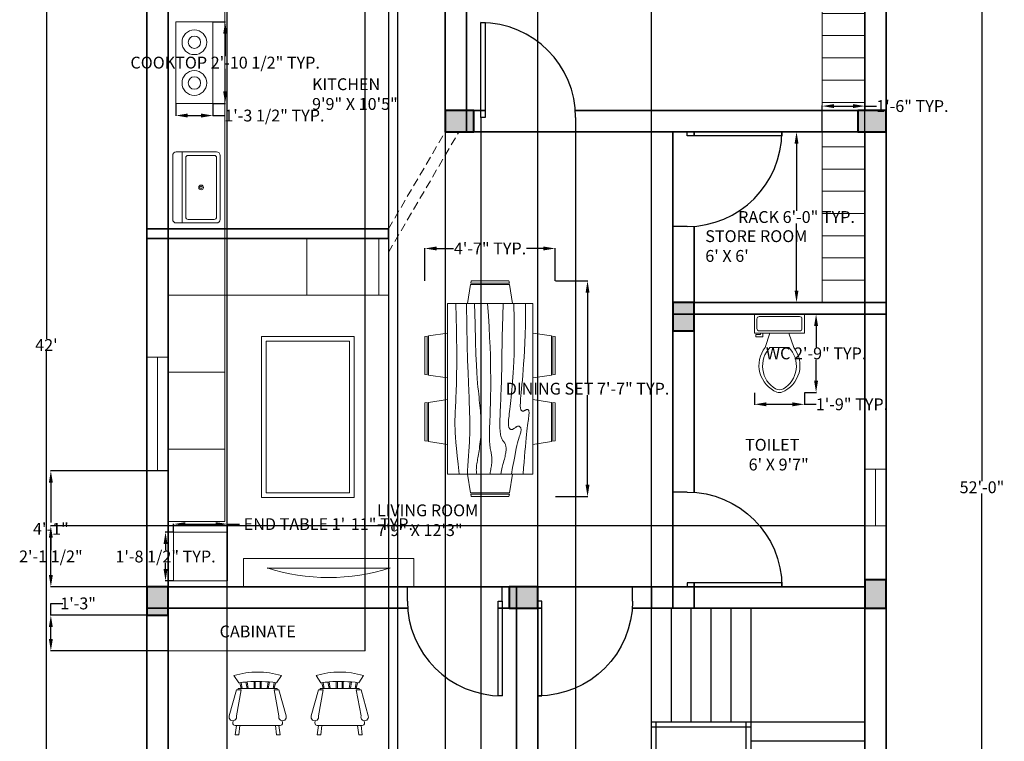
# Model space of a CAD drawing. Units: inches. Extents: x -54 to 881, y -122 to 681.
# Tile 2 of 6: x -54 to 362, y 205 to 509. Entities that reach past the tile are written whole.
import ezdxf

# ---------------------------------------------------------------- set-up
doc = ezdxf.new("R2010")
doc.units = ezdxf.units.IN
doc.header["$MEASUREMENT"] = 0
doc.linetypes.add('DASHED', pattern=[0.75, 0.5, -0.25])
for name, color, linetype, lineweight in [('A-ANNO-DIMS', 2, 'Continuous', 18), ('A-DOOR', 3, 'Continuous', 25), ('A-EQPM', 9, 'Continuous', 18), ('A-FLOR-CASE', 8, 'Continuous', 18), ('A-FLOR-FIXT', 9, 'Continuous', 18), ('A-FLOR-STRS', 7, 'Continuous', 25), ('A-FURN', 8, 'Continuous', 18), ('A-GLAZ', 4, 'Continuous', 20), ('A-WALL', 7, 'Continuous', 35), ('A-WALL-OVHD', 8, 'DASHED', 18)]:
    doc.layers.add(name, color=color, linetype=linetype, lineweight=lineweight)
for name, color, linetype, lineweight, true_color in [('A-ANNO-TEXT', 217, 'Continuous', 18, 0x93278f), ('A-AREA-IDEN', 217, 'Continuous', 18, 0x93278f), ('A-COLS', 240, 'Continuous', 40, 0xed1f24)]:
    doc.layers.add(name, color=color, linetype=linetype, lineweight=lineweight, true_color=true_color)
doc.styles.get("Standard").update_dxf_attribs({"font": 'arial.ttf'})
doc.dimstyles.get("Standard").update_dxf_attribs({"dimtxt": 5, "dimasz": 5, "dimexe": 0.18, "dimexo": 0.0625, "dimgap": 0.09, "dimtad": 0, "dimtih": 1, "dimtoh": 1, "dimdec": 0, "dimzin": 0, "dimdsep": 46, "dimlunit": 3, "dimtxsty": 'Standard', "dimcen": 0.09, "dimadec": 0, "dimazin": 0, "dimtfac": 1, "dimtdec": 0, "dimtofl": 0, "dimtmove": 0, "dimatfit": 3, "dimfxl": 1, "dimtolj": 1, "dimtzin": 0, "dimarcsym": 0})

# ---------------------------------------------------------------- blocks, each defined once
blk = doc.blocks.new('*D2')
at = {"layer": 'A-ANNO-DIMS', "color": 0, "lineweight": -2, "transparency": 16777216}
for p, q in [((-0.06, 624), (-42.51, 624)), ((-42.33, 619), (-42.33, 374.6)), ((-42.33, 125), (-42.33, 369.4)), ((-0.06, 120), (-42.51, 120))]:
    blk.add_line(p, q, dxfattribs=at)
at = {"layer": 'A-ANNO-DIMS', "color": 0, "transparency": 16777216}
for points in [[(-43.17, 619), (-41.5, 619), (-42.33, 624)], [(-43.17, 125), (-41.5, 125), (-42.33, 120)]]:
    blk.add_solid(points, dxfattribs=at)
at = {"layer": 'Defpoints', "color": 0, "transparency": 16777216}
for p in [(0, 624), (-42.33, 120), (0, 120)]:
    blk.add_point(p, dxfattribs=at)
at = {"layer": 'A-ANNO-DIMS', "color": 0, "transparency": 16777216, "insert": (-42.33, 372), "char_height": 5, "attachment_point": 5}
blk.add_mtext("\\A1;42'", dxfattribs=at)
blk = doc.blocks.new('Toilet - top')
for p, q in [((9.5, -6), (9.5, -2)), ((-8, -8.5), (-8, -8)), ((-7, -8), (-7, -9.5)), ((-4, -8), (-6, -14)), ((4, -8), (6, -14)), ((-10, -8.5), (-8, -8.5)), ((-10, -9.5), (-10, -8.5)), ((-7, -9.5), (-10, -9.5)), ((4, -14), (-4, -14))]:
    blk.add_line(p, q)
blk.add_lwpolyline([(10.5, -8), (10.5, 0), (-10.5, 0), (-10.5, -8)], close=True)
for points in [[(-9.5, -2), (-9.5, -6)], [(8.5, -1), (-8.5, -1)], [(-8.5, -7), (8.5, -7)]]:
    blk.add_lwpolyline(points)
for centre, radius, start, end in [((-8.62, -1.88), 0.884, 81.8699, 188.1301), ((8.62, -1.88), 0.884, 351.8699, 98.1301), ((-8.62, -6.12), 0.884, 171.8699, 278.1301), ((8.62, -6.12), 0.884, 261.8699, 8.1301), ((3.52, -21.58), 12.17, 141.4691, 247.9714), ((4.2, -21.82), 11.33, 136.3677, 238.9468), ((-3.52, -21.58), 12.17, 292.0284, 38.5307), ((-4.2, -21.82), 11.33, 301.053, 43.6321), ((0, -27.88), 4, 245.7318, 294.2682), ((0, -29), 4, 254.8605, 285.1395)]:
    blk.add_arc(centre, radius, start, end)
blk = doc.blocks.new('Sink-single - 30 in top')
blk.add_line((-15, -3.999996), (15, -3.999996))
for points in [[(-13.5, 0), (13.5, 0)], [(-15, -18.499996), (-15, -1.5)], [(15, -1.5), (15, -18.499996)], [(-13.5, -17.499996), (-13.5, -6.499996)], [(-12.5, -5.499996), (12.5, -5.499996)], [(13.5, -6.499996), (13.5, -17.499996)], [(13.5, -19.999996), (-13.5, -19.999996)], [(12.5, -18.499996), (-12.5, -18.499996)]]:
    blk.add_lwpolyline(points)
for radius in [1, 0.5]:
    blk.add_circle((0, -11.999996), radius)
for centre, radius, start, end in [((-13.5, -1.5), 1.5, 90, 180), ((13.5, -1.5), 1.5, 0, 90), ((-12.5, -6.499996), 1, 90, 180), ((12.5, -6.499996), 1, 0, 90), ((-13.5, -18.499996), 1.5, 180, 270), ((-12.5, -17.499996), 1, 180, 270), ((12.5, -17.499996), 1, 270, 0), ((13.5, -18.499996), 1.5, 270, 0)]:
    blk.add_arc(centre, radius, start, end)
blk = doc.blocks.new('Dining Set - 36 x 72 in.')
for p, q in [((-22.2343, 26.00059), (-23.4847, 17.99762)), ((-22.2304, 26), (-5.7608, 26)), ((-22, 27.5), (-22.1562, 26.50042)), ((-5.8416, 26.5), (-22.1534, 26.5)), ((-22, 27.5), (-6, 27.5)), ((-5.8437, 26.49966), (-6, 27.5)), ((-4.5152, 17.99762), (-5.7655, 25.99926)), ((5.7657, 26.00059), (4.5153, 17.99762)), ((5.7696, 26), (22.2392, 26)), ((6, 27.5), (5.8438, 26.50042)), ((22.1584, 26.5), (5.8466, 26.5)), ((6, 27.5), (22, 27.5)), ((22.1563, 26.49966), (22, 27.5)), ((23.4848, 17.99762), (22.2345, 25.99926)), ((36, 18), (-36, 18)), ((-36, 18), (-36, -18)), ((36, -18), (36, 18)), ((-44.0006, 8.23428), (-35.9976, 9.48474)), ((44.0006, 8.23428), (35.9976, 9.48474)), ((-45.5, 8), (-44.5004, 8.15617)), ((-45.5, 8), (-45.5, -8)), ((-44.5, -8.15843), (-44.5, 8.15338)), ((-44, 8.23041), (-44, -8.23915)), ((44, 8.23041), (44, -8.23915)), ((44.5, -8.15843), (44.5, 8.15338)), ((45.5, 8), (44.5005, 8.15617)), ((45.5, 8), (45.5, -8)), ((-44.4997, -8.15631), (-45.5, -8)), ((-35.9976, -9.48476), (-43.9993, -8.2345)), ((35.9976, -9.48476), (43.9993, -8.2345)), ((44.4997, -8.15631), (45.5, -8)), ((-36, -18), (36, -18)), ((-22.2343, -26.0006), (-23.4847, -17.99762)), ((-4.5152, -17.99762), (-5.7655, -25.99928)), ((5.7657, -26.0006), (4.5153, -17.99762)), ((23.4848, -17.99762), (22.2345, -25.99928)), ((-22.2304, -26), (-5.7608, -26)), ((-22, -27.5), (-22.1562, -26.50044)), ((-5.8416, -26.5), (-22.1534, -26.5)), ((-22, -27.5), (-6, -27.5)), ((-5.8437, -26.49967), (-6, -27.5)), ((5.7696, -26), (22.2392, -26)), ((6, -27.5), (5.8438, -26.50044)), ((22.1584, -26.5), (5.8466, -26.5)), ((6, -27.5), (22, -27.5)), ((22.1563, -26.49967), (22, -27.5))]:
    blk.add_line(p, q)
for points in [[(-36, 15), (-31.1772, 14.97754), (-26.8079, 14.91406), (-22.8538, 14.81543), (-19.276, 14.6875), (-16.0362, 14.53613), (-13.0957, 14.36718), (-10.4159, 14.18652), (-7.9583, 14), (-5.6904, 13.81315), (-3.6035, 13.63021), (-1.6954, 13.45508), (0.0365, 13.29166), (1.5945, 13.14388), (2.9811, 13.01562), (4.1988, 12.9108), (5.25, 12.83333), (6.1393, 12.78613), (6.8802, 12.76823), (7.4883, 12.77767), (7.9792, 12.8125), (8.3685, 12.87077), (8.6719, 12.95052), (8.9049, 13.0498), (9.0833, 13.16666), (9.2205, 13.29899), (9.3216, 13.44401), (9.3895, 13.59879), (9.4271, 13.76041), (9.4373, 13.92594), (9.4232, 14.09245), (9.3875, 14.257), (9.3333, 14.41666), (9.2638, 14.56917), (9.1836, 14.71484), (9.0975, 14.85465), (9.0104, 14.98958), (8.9272, 15.1206), (8.8529, 15.2487), (8.7922, 15.37483), (8.75, 15.5), (8.7305, 15.62467), (8.7344, 15.74739), (8.7617, 15.86621), (8.8125, 15.97916), (8.8867, 16.08431), (8.9844, 16.17968), (9.1055, 16.26334), (9.25, 16.33333), (9.4189, 16.38802), (9.6172, 16.42708), (9.8506, 16.45052), (10.125, 16.45833), (10.4463, 16.45052), (10.8203, 16.42708), (11.2529, 16.38802), (11.75, 16.33333), (12.3184, 16.26318), (12.9694, 16.17838), (13.7151, 16.07991), (14.5677, 15.96875), (15.5395, 15.84586), (16.6426, 15.71224), (17.8893, 15.56884), (19.2917, 15.41666), (20.859, 15.25667), (22.5879, 15.08984), (24.4721, 14.91715), (26.5052, 14.73958), (28.6809, 14.5581), (30.9929, 14.3737), (33.4347, 14.18733), (36, 14)], [(-36, 10), (-28.9766, 10.14274), (-23.1725, 10.20442), (-18.4241, 10.19775), (-14.5677, 10.13541), (-11.4399, 10.03011), (-8.877, 9.89453), (-6.7154, 9.74137), (-4.7917, 9.58333), (-2.9698, 9.43082), (-1.2246, 9.28515), (0.4415, 9.14534), (2.026, 9.01041), (3.5266, 8.87939), (4.9408, 8.7513), (6.266, 8.62516), (7.5, 8.5), (8.6411, 8.37549), (9.6914, 8.2539), (10.6538, 8.13818), (11.5312, 8.03125), (12.3267, 7.93603), (13.043, 7.85547), (13.6831, 7.79248), (14.25, 7.75), (14.7471, 7.7303), (15.1797, 7.73307), (15.5537, 7.75732), (15.875, 7.80208), (16.1494, 7.86637), (16.3828, 7.94922), (16.5811, 8.04964), (16.75, 8.16666), (16.8944, 8.29915), (17.0143, 8.44531), (17.1089, 8.60319), (17.1771, 8.77083), (17.218, 8.94629), (17.2305, 9.1276), (17.2137, 9.31282), (17.1667, 9.5), (17.0895, 9.6875), (16.987, 9.875), (16.8649, 10.0625), (16.7292, 10.25), (16.5856, 10.4375), (16.4401, 10.625), (16.2985, 10.8125), (16.1667, 11), (16.05, 11.18733), (15.9518, 11.3737), (15.8752, 11.5581), (15.8229, 11.73958), (15.798, 11.91715), (15.8034, 12.08984), (15.842, 12.25667), (15.9167, 12.41666), (16.0295, 12.56836), (16.1784, 12.70833), (16.3605, 12.83268), (16.5729, 12.9375), (16.8127, 13.01888), (17.0768, 13.07291), (17.3625, 13.0957), (17.6667, 13.08333), (17.9894, 13.03312), (18.3418, 12.94726), (18.7382, 12.82918), (19.1927, 12.68229), (19.7195, 12.51001), (20.3327, 12.31575), (21.0465, 12.10294), (21.875, 11.875), (22.8357, 11.63354), (23.959, 11.37304), (25.2786, 11.08618), (26.8282, 10.76562), (28.6414, 10.40405), (30.752, 9.99414), (33.1936, 9.52856), (36, 9)], [(-36, 5.5), (-30.7157, 5.3348), (-26.069, 5.20963), (-21.9946, 5.11767), (-18.4271, 5.05208), (-15.3009, 5.00602), (-12.5508, 4.97265), (-10.1112, 4.94515), (-7.9167, 4.91666), (-5.909, 4.88167), (-4.0586, 4.83984), (-2.3429, 4.79215), (-0.7396, 4.73958), (0.7739, 4.6831), (2.22, 4.6237), (3.6213, 4.56233), (5, 4.5), (6.373, 4.43782), (7.7344, 4.3776), (9.0723, 4.32129), (10.375, 4.27083), (11.6309, 4.22819), (12.8281, 4.19531), (13.9551, 4.17415), (15, 4.16666), (15.954, 4.17448), (16.819, 4.19791), (17.6001, 4.23698), (18.3021, 4.29166), (18.9299, 4.36198), (19.4883, 4.44791), (19.9823, 4.54948), (20.4167, 4.66666), (20.7969, 4.79899), (21.1302, 4.94401), (21.4245, 5.09879), (21.6875, 5.26041), (21.9271, 5.42594), (22.1511, 5.59245), (22.3672, 5.757), (22.5834, 5.91666), (22.8065, 6.06868), (23.0404, 6.21093), (23.2879, 6.34147), (23.5521, 6.45833), (23.8358, 6.55957), (24.142, 6.64323), (24.4735, 6.70735), (24.8334, 6.75), (25.2235, 6.76969), (25.642, 6.76692), (26.0858, 6.74267), (26.5521, 6.69791), (27.0379, 6.63362), (27.5404, 6.55078), (28.0565, 6.45036), (28.5834, 6.33333), (29.1242, 6.19987), (29.7071, 6.04687), (30.3661, 5.87044), (31.1354, 5.66666), (32.0493, 5.43164), (33.142, 5.16146), (34.4475, 4.85221), (36, 4.5)], [(-36, -1), (-30.7915, -0.6591), (-26.0195, -0.38216), (-21.6519, -0.16284), (-17.6563, 0.00521), (-14.0005, 0.12833), (-10.6523, 0.21289), (-7.5796, 0.26522), (-4.75, 0.29166), (-2.134, 0.29793), (0.2878, 0.28711), (2.5317, 0.26163), (4.6146, 0.22396), (6.5529, 0.17651), (8.3633, 0.12174), (10.0623, 0.06209), (11.6667, 0), (13.1899, -0.06201), (14.6341, -0.1211), (15.9982, -0.17432), (17.2813, -0.21875), (18.4823, -0.25147), (19.6003, -0.26953), (20.6343, -0.27002), (21.5834, -0.25), (22.4481, -0.20768), (23.2357, -0.14584), (23.9549, -0.06836), (24.6146, 0.02083), (25.2235, 0.11784), (25.7904, 0.21875), (26.3241, 0.31966), (26.8334, 0.41666), (27.3265, 0.50618), (27.8099, 0.58593), (28.2894, 0.65397), (28.7709, 0.70833), (29.2601, 0.74707), (29.763, 0.76823), (30.2855, 0.76985), (30.8334, 0.75), (31.4088, 0.70784), (31.9994, 0.64713), (32.589, 0.57275), (33.1615, 0.48958), (33.7008, 0.4025), (34.1908, 0.3164), (34.6153, 0.23616), (34.9584, 0.16666), (35.2099, 0.11165), (35.3848, 0.07031), (35.504, 0.04069), (35.5886, 0.02083), (35.6594, 0.00879), (35.7377, 0.0026), (35.8442, 0.00032), (36, 0)], [(-36, -6.5), (-27.1843, -6.31267), (-20.084, -6.1263), (-14.469, -5.9419), (-10.1094, -5.76042), (-6.7752, -5.58285), (-4.2363, -5.41016), (-2.2629, -5.24333), (-0.625, -5.08334), (0.8708, -4.93099), (2.2715, -4.78646), (3.5872, -4.64974), (4.8281, -4.52084), (6.0046, -4.39974), (7.127, -4.28646), (8.2053, -4.18099), (9.25, -4.08334), (10.2705, -3.99382), (11.2734, -3.91407), (12.2647, -3.84603), (13.25, -3.79167), (14.2354, -3.75293), (15.2266, -3.73177), (16.2295, -3.73015), (17.25, -3.75), (18.2912, -3.79248), (19.3451, -3.85547), (20.4009, -3.93604), (21.4479, -4.03125), (22.4754, -4.13819), (23.4727, -4.25391), (24.4289, -4.37549), (25.3334, -4.5), (26.1785, -4.62492), (26.9694, -4.74935), (27.7145, -4.87281), (28.4219, -4.99479), (29.1, -5.11483), (29.7572, -5.23242), (30.4016, -5.34709), (31.0417, -5.45834), (31.6837, -5.56437), (32.3262, -5.65821), (32.9658, -5.73153), (33.599, -5.77604), (34.2224, -5.78345), (34.8327, -5.74545), (35.4264, -5.65373), (36, -5.5)], [(-36, -10), (-26.4022, -9.81299), (-18.4675, -9.62891), (-11.9839, -9.45069), (-6.7396, -9.28125), (-2.5226, -9.12354), (0.8789, -8.98047), (3.6769, -8.85498), (6.0833, -8.75), (8.2767, -8.66765), (10.3021, -8.60677), (12.1712, -8.56543), (13.8958, -8.54167), (15.4876, -8.53353), (16.9583, -8.53907), (18.3197, -8.55632), (19.5834, -8.58334), (20.7616, -8.61841), (21.8685, -8.66081), (22.9188, -8.71004), (23.9271, -8.76563), (24.9081, -8.82707), (25.8763, -8.89388), (26.8465, -8.96558), (27.8334, -9.04167), (28.8474, -9.12118), (29.8828, -9.20117), (30.93, -9.27824), (31.9792, -9.34896), (33.0205, -9.40991), (34.0443, -9.45768), (35.0407, -9.48885), (36, -9.5)], [(-36, -14.5), (-30.0881, -14.33513), (-25.0332, -14.21224), (-20.7312, -14.12647), (-17.0781, -14.07292), (-13.97, -14.04671), (-11.3027, -14.04297), (-8.9724, -14.05681), (-6.875, -14.08334), (-4.9224, -14.11833), (-3.0905, -14.16016), (-1.3709, -14.20785), (0.2448, -14.26042), (1.7647, -14.3169), (3.1973, -14.3763), (4.5507, -14.43767), (5.8333, -14.5), (7.0554, -14.5621), (8.235, -14.62175), (9.3922, -14.67652), (10.5469, -14.72396), (11.7192, -14.76164), (12.929, -14.78711), (14.1965, -14.79794), (15.5417, -14.79167), (16.9933, -14.76424), (18.6152, -14.70508), (20.4804, -14.60197), (22.6615, -14.44271), (25.2312, -14.21509), (28.2624, -13.9069), (31.8277, -13.50594), (36, -13)]]:
    blk.add_lwpolyline(points)
blk = doc.blocks.new('*U12')
for p, q in [((0, 0), (0, -6)), ((40, 0), (40, -6))]:
    blk.add_line(p, q)
blk.add_lwpolyline([(0, 0), (0, 40), (1.75, 40), (1.75, 0)], close=True)
blk.add_arc((0, 0), 40, 0, 90)
blk = doc.blocks.new('Chair - Rocking')
for p, q in [((-8, -4.5), (-10, -1.5)), ((-1.5, -4.05012), (-1.5, -7)), ((-1, -7), (-1, -4.05012)), ((1, -7), (1, -4.04655)), ((1.5, -4.05012), (1.5, -7)), ((8, -4.5), (10, -1.5)), ((-9, -7.5), (-12, -18.49999)), ((-7, -7.5), (-9, -7.5)), ((-9, -18.49999), (-7, -7.5)), ((-8.23428, -6.99939), (-8.3093, -7.47958)), ((-8.23041, -7), (8.23915, -7)), ((-7.5, -4.5), (-7, -7)), ((-6.5, -7), (-7.02225, -4.43)), ((-4.5, -7), (-4.96674, -4.19951)), ((-4, -7), (-4.40532, -4.16272)), ((4, -7), (4.40187, -4.18694)), ((4.5, -7), (4.96761, -4.19437)), ((6.5, -7), (7, -4.4057)), ((7.5, -4.5), (7, -7)), ((7, -7.5), (9, -7.5)), ((9, -18.49999), (7, -7.5)), ((8.31071, -7.48854), (8.23449, -7.00073)), ((9, -7.5), (12, -18.49999)), ((-10.36644, -20.64523), (-10.5, -21.49999)), ((10.5, -21.49999), (10.3575, -20.58798)), ((-9, -22.49999), (-9.5, -26.49999)), ((0, -22.49999), (-9.5, -22.49999)), ((-8, -26.49999), (-7.5, -22.49999)), ((0, -22.49999), (9.5, -22.49999)), ((8, -26.49999), (7.5, -22.49999)), ((9, -22.49999), (9.5, -26.49999)), ((-9.5, -26.49999), (-8, -26.49999)), ((9.5, -26.49999), (8, -26.49999))]:
    blk.add_line(p, q)
for centre, radius, start, end in [((0, -34.08333), 34.08333, 72.93847, 107.0615), ((0, -68.25004), 64.25, 93.92211, 97.15267), ((0, -68.25004), 64.25, 82.84733, 93.92211), ((-10.5, -18.99999), 1.58114, 161.5651, 18.43495), ((10.5, -18.99999), 1.58114, 161.5651, 18.43495), ((-9.5, -21.49999), 1, 180, 270), ((9.5, -21.49999), 1, 270, 0)]:
    blk.add_arc(centre, radius, start, end)
blk = doc.blocks.new('WIN-48X9')
for p, q in [((0, 0), (0, 9)), ((48, 0), (48, 9)), ((0, 4.5), (48, 4.5))]:
    blk.add_line(p, q)
blk = doc.blocks.new('WIN-24X9')
for p, q in [((0, 24), (9, 24)), ((4.5, 24), (4.5, 0)), ((0, 0), (9, 0))]:
    blk.add_line(p, q)
blk = doc.blocks.new('COOKTOP-2-BURNER')
blk.add_lwpolyline([(0, 34.35), (15.67, 34.35), (15.67, 0), (0, 0)], close=True)
for centre, radius in [((7.83, 25.76), 5.22), ((7.83, 25.76), 2.61), ((7.83, 8.59), 5.22), ((7.83, 8.59), 2.61)]:
    blk.add_circle(centre, radius)
blk = doc.blocks.new('TV-52-PLAN')
blk.add_line((0, 4), (52, 4))
blk.add_arc((26, 86.41), 86.41, 252.4883, 287.5117)
blk = doc.blocks.new('LIVING-COFFEE-TABLE')
for points in [[(0, 67.86), (39.15, 67.86), (39.15, 0), (0, 0)], [(2, 65.86), (37.15, 65.86), (37.15, 2), (2, 2)]]:
    blk.add_lwpolyline(points, close=True)
blk = doc.blocks.new('STAIR-RETURN-FLIGHT')
for p, q in [((48, 93), (48, 141)), ((56.4, 93), (56.4, 141)), ((64.8, 93), (64.8, 141)), ((73.2, 93), (73.2, 141)), ((81.6, 93), (81.6, 141)), ((90, 93), (90, 141)), ((48, 0), (48, 93)), ((48, 93), (90, 93)), ((50, 0), (50, 93)), ((88, 0), (88, 93)), ((90, 0), (90, 93)), ((90, 93), (138, 93)), ((48, 91), (90, 91)), ((90, 85), (138, 85)), ((90, 77), (138, 77)), ((90, 69), (138, 69)), ((90, 61), (138, 61)), ((0, 57), (48, 57)), ((90, 53), (138, 53)), ((0, 49), (48, 49)), ((90, 45), (138, 45)), ((0, 41), (48, 41)), ((90, 37), (138, 37)), ((0, 33), (48, 33)), ((0, 25), (48, 25)), ((90, 29), (138, 29)), ((90, 21), (138, 21)), ((0, 17), (48, 17)), ((90, 13), (138, 13)), ((0, 9), (48, 9)), ((48, 2), (90, 2)), ((48, 0), (90, 0))]:
    blk.add_line(p, q)
blk = doc.blocks.new('KITCHEN-COUNTER-L')
for p, q in [((48, 101), (48, 125)), ((0, 0), (0, 101)), ((0, 101), (48, 101))]:
    blk.add_line(p, q)
blk = doc.blocks.new('STORAGE-RACK-144X18')
for p, q in [((0, 144), (18, 144)), ((0, 0), (0, 144)), ((0, 134.625), (18, 134.625)), ((0, 125.25), (18, 125.25)), ((0, 115.875), (18, 115.875)), ((0, 106.5), (18, 106.5)), ((0, 97.125), (18, 97.125)), ((0, 87.75), (18, 87.75)), ((0, 78.375), (18, 78.375)), ((0, 69), (18, 69)), ((0, 59.625), (18, 59.625)), ((0, 50.25), (18, 50.25)), ((0, 40.875), (18, 40.875)), ((0, 31.5), (18, 31.5)), ((0, 22.125), (18, 22.125)), ((0, 12.75), (18, 12.75)), ((0, 3.375), (18, 3.375))]:
    blk.add_line(p, q)
blk = doc.blocks.new('STORAGE-RACK-72X18')
for p, q in [((0, 0), (0, 72)), ((0, 65.625), (18, 65.625)), ((0, 56.25), (18, 56.25)), ((0, 46.875), (18, 46.875)), ((0, 37.5), (18, 37.5)), ((0, 28.125), (18, 28.125)), ((0, 18.75), (18, 18.75)), ((0, 9.375), (18, 9.375)), ((0, 0), (18, 0))]:
    blk.add_line(p, q)
blk = doc.blocks.new('COL-9X12')
h = blk.add_hatch(color=256)
h.dxf.hatch_style = 1
h.paths.add_polyline_path([(9, 12), (0, 12), (0, 0), (9, 0)])
blk.add_lwpolyline([(0, 0), (9, 0), (9, 12), (0, 12)], close=True)
blk = doc.blocks.new('LIVING-SIDE-TABLE')
blk.add_lwpolyline([(0, 20.5), (22.77, 20.5), (22.77, 0), (0, 0)], close=True)
blk = doc.blocks.new('*D54')
at = {"layer": 'A-ANNO-DIMS', "color": 0, "lineweight": -2, "transparency": 16777216}
for p, q in [((277.56, 385), (282.64, 385)), ((282.46, 380), (282.46, 371.15)), ((282.46, 356.95), (282.46, 365.8)), ((277.56, 351.95), (282.64, 351.95))]:
    blk.add_line(p, q, dxfattribs=at)
at = {"layer": 'A-ANNO-DIMS', "color": 0, "transparency": 16777216}
for points in [[(281.62, 380), (283.29, 380), (282.46, 385)], [(281.62, 356.95), (283.29, 356.95), (282.46, 351.95)]]:
    blk.add_solid(points, dxfattribs=at)
at = {"layer": 'Defpoints', "color": 0, "transparency": 16777216}
for p in [(277.5, 385), (282.46, 385), (277.5, 351.95)]:
    blk.add_point(p, dxfattribs=at)
at = {"layer": 'A-ANNO-DIMS', "color": 0, "transparency": 16777216, "insert": (282.46, 368.48), "char_height": 5, "attachment_point": 5}
blk.add_mtext('\\A1;WC 2\'-9" TYP.', dxfattribs=at)
blk = doc.blocks.new('*D55')
at = {"layer": 'A-ANNO-DIMS', "color": 0, "lineweight": -2, "transparency": 16777216}
for p, q in [((256.5, 351.89), (256.5, 346.82)), ((277.5, 351.89), (277.5, 346.82)), ((261.5, 347), (272.5, 347)), ((277.5, 347), (282.5, 347))]:
    blk.add_line(p, q, dxfattribs=at)
at = {"layer": 'A-ANNO-DIMS', "color": 0, "transparency": 16777216}
for points in [[(261.5, 347.83), (261.5, 346.16), (256.5, 347)], [(272.5, 347.83), (272.5, 346.16), (277.5, 347)]]:
    blk.add_solid(points, dxfattribs=at)
at = {"layer": 'Defpoints', "color": 0, "transparency": 16777216}
for p in [(256.5, 351.95), (277.5, 351.95), (277.5, 347)]:
    blk.add_point(p, dxfattribs=at)
at = {"layer": 'A-ANNO-DIMS', "color": 0, "transparency": 16777216, "insert": (297.59, 347), "char_height": 5, "attachment_point": 5}
blk.add_mtext('\\A1;1\'-9" TYP.', dxfattribs=at)
blk = doc.blocks.new('*D58')
at = {"layer": 'A-ANNO-DIMS', "color": 0, "lineweight": -2, "transparency": 16777216}
for p, q in [((172.43, 399.09), (186.2, 399.09)), ((186.02, 394.09), (186.02, 356.26)), ((186.02, 313.09), (186.02, 350.91)), ((172.43, 308.09), (186.2, 308.09))]:
    blk.add_line(p, q, dxfattribs=at)
at = {"layer": 'A-ANNO-DIMS', "color": 0, "transparency": 16777216}
for points in [[(185.19, 394.09), (186.85, 394.09), (186.02, 399.09)], [(185.19, 313.09), (186.85, 313.09), (186.02, 308.09)]]:
    blk.add_solid(points, dxfattribs=at)
at = {"layer": 'Defpoints', "color": 0, "transparency": 16777216}
for p in [(172.37, 399.09), (172.37, 308.09), (186.02, 308.09)]:
    blk.add_point(p, dxfattribs=at)
at = {"layer": 'A-ANNO-DIMS', "color": 0, "transparency": 16777216, "insert": (186.02, 353.59), "char_height": 5, "attachment_point": 5}
blk.add_mtext('\\A1;DINING SET 7\'-7" TYP.', dxfattribs=at)
blk = doc.blocks.new('*D59')
at = {"layer": 'A-ANNO-DIMS', "color": 0, "lineweight": -2, "transparency": 16777216}
for p, q in [((117.37, 399.15), (117.37, 412.92)), ((122.37, 412.74), (129.44, 412.74)), ((167.37, 412.74), (160.3, 412.74)), ((172.37, 399.15), (172.37, 412.92))]:
    blk.add_line(p, q, dxfattribs=at)
at = {"layer": 'A-ANNO-DIMS', "color": 0, "transparency": 16777216}
for points in [[(122.37, 413.57), (122.37, 411.9), (117.37, 412.74)], [(167.37, 413.57), (167.37, 411.9), (172.37, 412.74)]]:
    blk.add_solid(points, dxfattribs=at)
at = {"layer": 'Defpoints', "color": 0, "transparency": 16777216}
for p in [(172.37, 412.74), (117.37, 399.09), (172.37, 399.09)]:
    blk.add_point(p, dxfattribs=at)
at = {"layer": 'A-ANNO-DIMS', "color": 0, "transparency": 16777216, "insert": (144.87, 412.74), "char_height": 5, "attachment_point": 5}
blk.add_mtext('\\A1;4\'-7" TYP.', dxfattribs=at)
blk = doc.blocks.new('*D60')
at = {"layer": 'A-ANNO-DIMS', "color": 0, "lineweight": -2, "transparency": 16777216}
for p, q in [((28.02, 508.3), (33.29, 508.3)), ((33.11, 503.3), (33.11, 493.81)), ((33.11, 478.95), (33.11, 488.45)), ((28.02, 473.95), (33.29, 473.95))]:
    blk.add_line(p, q, dxfattribs=at)
at = {"layer": 'A-ANNO-DIMS', "color": 0, "transparency": 16777216}
for points in [[(32.27, 503.3), (33.94, 503.3), (33.11, 508.3)], [(32.27, 478.95), (33.94, 478.95), (33.11, 473.95)]]:
    blk.add_solid(points, dxfattribs=at)
at = {"layer": 'Defpoints', "color": 0, "transparency": 16777216}
for p in [(27.95, 508.3), (33.11, 508.3), (27.95, 473.95)]:
    blk.add_point(p, dxfattribs=at)
at = {"layer": 'A-ANNO-DIMS', "color": 0, "transparency": 16777216, "insert": (33.11, 491.13), "char_height": 5, "attachment_point": 5}
blk.add_mtext('\\A1;COOKTOP 2\'-10 1/2" TYP.', dxfattribs=at)
blk = doc.blocks.new('*D61')
at = {"layer": 'A-ANNO-DIMS', "color": 0, "lineweight": -2, "transparency": 16777216}
for p, q in [((12.29, 473.89), (12.29, 468.62)), ((27.95, 473.89), (27.95, 468.62)), ((17.29, 468.8), (22.95, 468.8)), ((27.95, 468.8), (32.95, 468.8))]:
    blk.add_line(p, q, dxfattribs=at)
at = {"layer": 'A-ANNO-DIMS', "color": 0, "transparency": 16777216}
for points in [[(17.29, 469.64), (17.29, 467.97), (12.29, 468.8)], [(22.95, 469.64), (22.95, 467.97), (27.95, 468.8)]]:
    blk.add_solid(points, dxfattribs=at)
at = {"layer": 'Defpoints', "color": 0, "transparency": 16777216}
for p in [(12.29, 473.95), (27.95, 473.95), (27.95, 468.8)]:
    blk.add_point(p, dxfattribs=at)
at = {"layer": 'A-ANNO-DIMS', "color": 0, "transparency": 16777216, "insert": (53.87, 468.8), "char_height": 5, "attachment_point": 5}
blk.add_mtext('\\A1;1\'-3 1/2" TYP.', dxfattribs=at)
blk = doc.blocks.new('*D70')
at = {"layer": 'A-ANNO-DIMS', "color": 0, "lineweight": -2, "transparency": 16777216}
for p, q in [((284.94, 462), (274.02, 462)), ((274.2, 457), (274.2, 428.68)), ((274.2, 395), (274.2, 423.32)), ((284.94, 390), (274.02, 390))]:
    blk.add_line(p, q, dxfattribs=at)
at = {"layer": 'A-ANNO-DIMS', "color": 0, "transparency": 16777216}
for points in [[(273.37, 457), (275.03, 457), (274.2, 462)], [(273.37, 395), (275.03, 395), (274.2, 390)]]:
    blk.add_solid(points, dxfattribs=at)
at = {"layer": 'Defpoints', "color": 0, "transparency": 16777216}
for p in [(274.2, 462), (285, 462), (285, 390)]:
    blk.add_point(p, dxfattribs=at)
at = {"layer": 'A-ANNO-DIMS', "color": 0, "transparency": 16777216, "insert": (274.2, 426), "char_height": 5, "attachment_point": 5}
blk.add_mtext('\\A1;RACK 6\'-0" TYP.', dxfattribs=at)
blk = doc.blocks.new('*D71')
at = {"layer": 'A-ANNO-DIMS', "color": 0, "lineweight": -2, "transparency": 16777216}
for p, q in [((285, 462.06), (285, 472.98)), ((290, 472.8), (298, 472.8)), ((303, 462.06), (303, 472.98)), ((303, 472.8), (308, 472.8))]:
    blk.add_line(p, q, dxfattribs=at)
at = {"layer": 'A-ANNO-DIMS', "color": 0, "transparency": 16777216}
for points in [[(290, 473.63), (290, 471.97), (285, 472.8)], [(298, 473.63), (298, 471.97), (303, 472.8)]]:
    blk.add_solid(points, dxfattribs=at)
at = {"layer": 'Defpoints', "color": 0, "transparency": 16777216}
for p in [(303, 472.8), (285, 462), (303, 462)]:
    blk.add_point(p, dxfattribs=at)
at = {"layer": 'A-ANNO-DIMS', "color": 0, "transparency": 16777216, "insert": (323.09, 472.8), "char_height": 5, "attachment_point": 5}
blk.add_mtext('\\A1;1\'-6" TYP.', dxfattribs=at)
blk = doc.blocks.new('*D72')
at = {"layer": 'A-ANNO-DIMS', "color": 0, "lineweight": -2, "transparency": 16777216}
for p, q in [((11.35, 293.1), (11.35, 296.64)), ((16.35, 296.46), (29.13, 296.46)), ((34.13, 293.1), (34.13, 296.64)), ((34.13, 296.46), (39.13, 296.46))]:
    blk.add_line(p, q, dxfattribs=at)
at = {"layer": 'A-ANNO-DIMS', "color": 0, "transparency": 16777216}
for points in [[(16.35, 297.29), (16.35, 295.62), (11.35, 296.46)], [(29.13, 297.29), (29.13, 295.62), (34.13, 296.46)]]:
    blk.add_solid(points, dxfattribs=at)
at = {"layer": 'Defpoints', "color": 0, "transparency": 16777216}
for p in [(34.13, 296.46), (11.35, 293.04), (34.13, 293.04)]:
    blk.add_point(p, dxfattribs=at)
at = {"layer": 'A-ANNO-DIMS', "color": 0, "transparency": 16777216, "insert": (76.65, 296.46), "char_height": 5, "attachment_point": 5}
blk.add_mtext('\\A1;END TABLE 1\'-11" TYP.', dxfattribs=at)
blk = doc.blocks.new('*D73')
at = {"layer": 'A-ANNO-DIMS', "color": 0, "lineweight": -2, "transparency": 16777216}
for p, q in [((11.29, 293.04), (7.76, 293.04)), ((7.94, 288.04), (7.94, 285.47)), ((7.94, 277.54), (7.94, 280.12)), ((11.29, 272.54), (7.76, 272.54))]:
    blk.add_line(p, q, dxfattribs=at)
at = {"layer": 'A-ANNO-DIMS', "color": 0, "transparency": 16777216}
for points in [[(7.1, 288.04), (8.77, 288.04), (7.94, 293.04)], [(7.1, 277.54), (8.77, 277.54), (7.94, 272.54)]]:
    blk.add_solid(points, dxfattribs=at)
at = {"layer": 'Defpoints', "color": 0, "transparency": 16777216}
for p in [(7.94, 293.04), (11.35, 293.04), (11.35, 272.54)]:
    blk.add_point(p, dxfattribs=at)
at = {"layer": 'A-ANNO-DIMS', "color": 0, "transparency": 16777216, "insert": (7.94, 282.79), "char_height": 5, "attachment_point": 5}
blk.add_mtext('\\A1;1\'-8 1/2" TYP.', dxfattribs=at)
blk = doc.blocks.new('*D74')
at = {"layer": 'A-ANNO-DIMS', "color": 0, "lineweight": -2, "transparency": 16777216}
for p, q in [((312.06, 624), (352.63, 624)), ((352.45, 619), (352.45, 314.64)), ((352.45, 5), (352.45, 309.36)), ((312.06, 0), (352.63, 0))]:
    blk.add_line(p, q, dxfattribs=at)
at = {"layer": 'A-ANNO-DIMS', "color": 0, "transparency": 16777216}
for points in [[(351.62, 619), (353.28, 619), (352.45, 624)], [(351.62, 5), (353.28, 5), (352.45, 0)]]:
    blk.add_solid(points, dxfattribs=at)
at = {"layer": 'Defpoints', "color": 0, "transparency": 16777216}
for p in [(312, 624), (352.45, 624), (312, 0)]:
    blk.add_point(p, dxfattribs=at)
at = {"layer": 'A-ANNO-DIMS', "color": 0, "transparency": 16777216, "insert": (352.45, 312), "char_height": 5, "attachment_point": 5}
blk.add_mtext('\\A1;52\'-0"', dxfattribs=at)
blk = doc.blocks.new('*D76')
at = {"layer": 'A-ANNO-DIMS', "color": 0, "lineweight": -2, "transparency": 16777216}
for p, q in [((126, 548.94), (126, -40.63)), ((102, 545.94), (102, -40.63)), ((107, -40.45), (107.22, -40.45)), ((121, -40.45), (120.78, -40.45))]:
    blk.add_line(p, q, dxfattribs=at)
at = {"layer": 'A-ANNO-DIMS', "color": 0, "transparency": 16777216}
for points in [[(107, -39.62), (107, -41.28), (102, -40.45)], [(121, -39.62), (121, -41.28), (126, -40.45)]]:
    blk.add_solid(points, dxfattribs=at)
at = {"layer": 'Defpoints', "color": 0, "transparency": 16777216}
for p in [(126, 549), (102, 546), (126, -40.45)]:
    blk.add_point(p, dxfattribs=at)
at = {"layer": 'A-ANNO-DIMS', "color": 0, "transparency": 16777216, "insert": (114, -40.45), "char_height": 5, "attachment_point": 5}
blk.add_mtext('\\A1;2\'-0"', dxfattribs=at)
blk = doc.blocks.new('*D77')
at = {"layer": 'A-ANNO-DIMS', "color": 0, "lineweight": -2, "transparency": 16777216}
for p, q in [((141, 461.94), (141, -40.63)), ((181, 461.94), (181, -40.63)), ((146, -40.45), (154.27, -40.45)), ((176, -40.45), (167.73, -40.45))]:
    blk.add_line(p, q, dxfattribs=at)
at = {"layer": 'A-ANNO-DIMS', "color": 0, "transparency": 16777216}
for points in [[(146, -39.62), (146, -41.28), (141, -40.45)], [(176, -39.62), (176, -41.28), (181, -40.45)]]:
    blk.add_solid(points, dxfattribs=at)
at = {"layer": 'Defpoints', "color": 0, "transparency": 16777216}
for p in [(141, 462), (181, 462), (181, -40.45)]:
    blk.add_point(p, dxfattribs=at)
at = {"layer": 'A-ANNO-DIMS', "color": 0, "transparency": 16777216, "insert": (161, -40.45), "char_height": 5, "attachment_point": 5}
blk.add_mtext('\\A1;3\'-4"', dxfattribs=at)
blk = doc.blocks.new('*D82')
at = {"layer": 'A-ANNO-DIMS', "color": 0, "lineweight": -2, "transparency": 16777216}
for p, q in [((302.94, 295.69), (-40.63, 295.69)), ((-40.45, 290.69), (-40.45, 285.52)), ((-40.45, 275), (-40.45, 280.17)), ((302.94, 270), (-40.63, 270))]:
    blk.add_line(p, q, dxfattribs=at)
at = {"layer": 'A-ANNO-DIMS', "color": 0, "transparency": 16777216}
for points in [[(-41.28, 290.69), (-39.62, 290.69), (-40.45, 295.69)], [(-41.28, 275), (-39.62, 275), (-40.45, 270)]]:
    blk.add_solid(points, dxfattribs=at)
at = {"layer": 'Defpoints', "color": 0, "transparency": 16777216}
for p in [(-40.45, 295.69), (303, 295.69), (303, 270)]:
    blk.add_point(p, dxfattribs=at)
at = {"layer": 'A-ANNO-DIMS', "color": 0, "transparency": 16777216, "insert": (-40.45, 282.84), "char_height": 5, "attachment_point": 5}
blk.add_mtext('\\A1;2\'-1 1/2"', dxfattribs=at)
blk = doc.blocks.new('*D83')
at = {"layer": 'A-ANNO-DIMS', "color": 0, "lineweight": -2, "transparency": 16777216}
for p, q in [((8.94, 318.95), (-40.63, 318.95)), ((-40.45, 313.95), (-40.45, 297.08)), ((-40.45, 275), (-40.45, 291.87)), ((8.94, 270), (-40.63, 270))]:
    blk.add_line(p, q, dxfattribs=at)
at = {"layer": 'A-ANNO-DIMS', "color": 0, "transparency": 16777216}
for points in [[(-41.28, 313.95), (-39.62, 313.95), (-40.45, 318.95)], [(-41.28, 275), (-39.62, 275), (-40.45, 270)]]:
    blk.add_solid(points, dxfattribs=at)
at = {"layer": 'Defpoints', "color": 0, "transparency": 16777216}
for p in [(-40.45, 318.95), (9, 318.95), (9, 270)]:
    blk.add_point(p, dxfattribs=at)
at = {"layer": 'A-ANNO-DIMS', "color": 0, "transparency": 16777216, "insert": (-40.45, 294.48), "char_height": 5, "attachment_point": 5}
blk.add_mtext('\\A1;4\'-1"', dxfattribs=at)
blk = doc.blocks.new('*D85')
at = {"layer": 'A-ANNO-DIMS', "color": 0, "lineweight": -2, "transparency": 16777216}
for p, q in [((33.99, 120.06), (33.99, 664.63)), ((38.99, 664.45), (63.24, 664.45)), ((100.99, 664.45), (76.73, 664.45)), ((105.99, 120.06), (105.99, 664.63))]:
    blk.add_line(p, q, dxfattribs=at)
at = {"layer": 'A-ANNO-DIMS', "color": 0, "transparency": 16777216}
for points in [[(38.99, 665.28), (38.99, 663.62), (33.99, 664.45)], [(100.99, 665.28), (100.99, 663.62), (105.99, 664.45)]]:
    blk.add_solid(points, dxfattribs=at)
at = {"layer": 'Defpoints', "color": 0, "transparency": 16777216}
for p in [(105.99, 664.45), (33.99, 120), (105.99, 120)]:
    blk.add_point(p, dxfattribs=at)
at = {"layer": 'A-ANNO-DIMS', "color": 0, "transparency": 16777216, "insert": (69.99, 664.45), "char_height": 5, "attachment_point": 5}
blk.add_mtext('\\A1;6\'-0"', dxfattribs=at)
blk = doc.blocks.new('*D89')
at = {"layer": 'A-ANNO-DIMS', "color": 0, "lineweight": -2, "transparency": 16777216}
for p, q in [((165, 120.06), (165, 664.63)), ((170, 664.45), (182.16, 664.45)), ((208, 664.45), (195.84, 664.45)), ((213, 120.06), (213, 664.63))]:
    blk.add_line(p, q, dxfattribs=at)
at = {"layer": 'A-ANNO-DIMS', "color": 0, "transparency": 16777216}
for points in [[(170, 665.28), (170, 663.62), (165, 664.45)], [(208, 665.28), (208, 663.62), (213, 664.45)]]:
    blk.add_solid(points, dxfattribs=at)
at = {"layer": 'Defpoints', "color": 0, "transparency": 16777216}
for p in [(213, 664.45), (165, 120), (213, 120)]:
    blk.add_point(p, dxfattribs=at)
at = {"layer": 'A-ANNO-DIMS', "color": 0, "transparency": 16777216, "insert": (189, 664.45), "char_height": 5, "attachment_point": 5}
blk.add_mtext('\\A1;4\'-0"', dxfattribs=at)
blk = doc.blocks.new('*D90')
at = {"layer": 'A-ANNO-DIMS', "color": 0, "lineweight": -2, "transparency": 16777216}
for p, q in [((9, 243.06), (9, 664.63)), ((14, 664.45), (41.88, 664.45)), ((87.14, 664.45), (59.26, 664.45)), ((92.14, 243.06), (92.14, 664.63))]:
    blk.add_line(p, q, dxfattribs=at)
at = {"layer": 'A-ANNO-DIMS', "color": 0, "transparency": 16777216}
for points in [[(14, 665.28), (14, 663.62), (9, 664.45)], [(87.14, 665.28), (87.14, 663.62), (92.14, 664.45)]]:
    blk.add_solid(points, dxfattribs=at)
at = {"layer": 'Defpoints', "color": 0, "transparency": 16777216}
for p in [(92.14, 664.45), (9, 243), (92.14, 243)]:
    blk.add_point(p, dxfattribs=at)
at = {"layer": 'A-ANNO-DIMS', "color": 0, "transparency": 16777216, "insert": (50.57, 664.45), "char_height": 5, "attachment_point": 5}
blk.add_mtext('\\A1;6\'-11"', dxfattribs=at)
blk = doc.blocks.new('*D91')
at = {"layer": 'A-ANNO-DIMS', "color": 0, "lineweight": -2, "transparency": 16777216}
for p, q in [((-40.45, 258), (-40.45, 263)), ((-40.45, 263), (-35.45, 263)), ((8.94, 258), (-40.63, 258)), ((-40.45, 248), (-40.45, 253)), ((8.94, 243), (-40.63, 243))]:
    blk.add_line(p, q, dxfattribs=at)
at = {"layer": 'A-ANNO-DIMS', "color": 0, "transparency": 16777216}
for points in [[(-41.28, 253), (-39.62, 253), (-40.45, 258)], [(-41.28, 248), (-39.62, 248), (-40.45, 243)]]:
    blk.add_solid(points, dxfattribs=at)
at = {"layer": 'Defpoints', "color": 0, "transparency": 16777216}
for p in [(-40.45, 258), (9, 258), (9, 243)]:
    blk.add_point(p, dxfattribs=at)
at = {"layer": 'A-ANNO-DIMS', "color": 0, "transparency": 16777216, "insert": (-28.95, 263), "char_height": 5, "attachment_point": 5}
blk.add_mtext('\\A1;1\'-3"', dxfattribs=at)

msp = doc.modelspace()

# ---------------------------------------------------------------- linework, layer by layer
at = {"layer": 'A-FLOR-CASE'}
for p, q in [((92.14, 243), (92.14, 261)), ((9, 243), (92.14, 243))]:
    msp.add_line(p, q, dxfattribs=at)
at = {"layer": 'A-FURN'}
for p, q in [((33, 297.51), (33, 421)), ((33, 417), (102, 417)), ((67.5, 417), (67.5, 393)), ((98, 393), (98, 417)), ((102, 393), (102, 417)), ((9, 393), (33, 393)), ((33, 393), (102, 393)), ((9, 360.55), (33, 360.55)), ((9, 328.1), (33, 328.1)), ((9, 297.51), (33, 297.51)), ((40.78, 270), (40.78, 282)), ((40.78, 282), (112.78, 282)), ((112.78, 282), (112.78, 270))]:
    msp.add_line(p, q, dxfattribs=at)
at = {"layer": 'A-WALL'}
for p, q in [((0, 0), (0, 624)), ((126, 462), (126, 624)), ((135, 462), (135, 624)), ((312, 0), (312, 624)), ((303, 471), (303, 615)), ((9, 421), (9, 546)), ((135, 471), (142.75, 471)), ((180.89, 471), (312, 471)), ((135, 462), (126, 462)), ((135, 462), (312, 462)), ((222, 261), (222, 462)), ((231, 460.25), (231, 462)), ((303, 390), (303, 462)), ((0, 421), (102, 421)), ((9, 270), (9, 421)), ((102, 421), (102, 417)), ((231, 309.89), (231, 422.11)), ((0, 417), (102, 417)), ((222, 390), (312, 390)), ((303, 0), (303, 390)), ((222, 385), (312, 385)), ((231, 261), (231, 271.75)), ((0, 270), (303, 270)), ((9, 120), (9, 270)), ((156, 168.89), (156, 270)), ((165, 120), (165, 270)), ((213, 261), (213, 270)), ((0, 261), (110.11, 261)), ((148.25, 261), (166.75, 261)), ((204.89, 261), (303, 261))]:
    msp.add_line(p, q, dxfattribs=at)
at = {"layer": 'A-WALL-OVHD', "ltscale": 7}
for p, q in [((102, 421), (126, 462)), ((102, 411.1), (131.79, 462))]:
    msp.add_line(p, q, dxfattribs=at)

# ---------------------------------------------------------------- block references
at = {"layer": 'A-COLS'}
for p, rotation in [((126, 471), 270), ((300, 471), 270), ((165, 261), 90)]:
    msp.add_blockref('COL-9X12', p, dxfattribs=dict(at, rotation=rotation))
for p in [(222, 378), (303, 261), (0, 258)]:
    msp.add_blockref('COL-9X12', p, dxfattribs=at)
at = {"layer": 'A-DOOR'}
msp.add_blockref('*U12', (141, 468), dxfattribs=at)
for p, rotation in [((228, 462), 270), ((150, 264), 180)]:
    msp.add_blockref('*U12', p, dxfattribs=dict(at, rotation=rotation))
at = {"layer": 'A-DOOR', "xscale": -1}
for p, rotation in [((228, 270), 270), ((165, 264), 180)]:
    msp.add_blockref('*U12', p, dxfattribs=dict(at, rotation=rotation))
at = {"layer": 'A-EQPM'}
for name, p in [('COOKTOP-2-BURNER', (12.29, 473.95)), ('TV-52-PLAN', (50.78, 273.95))]:
    msp.add_blockref(name, p, dxfattribs=at)
at = {"layer": 'A-FLOR-CASE'}
for name, p in [('STORAGE-RACK-144X18', (285, 471)), ('KITCHEN-COUNTER-L', (33, 421)), ('STORAGE-RACK-72X18', (285, 390))]:
    msp.add_blockref(name, p, dxfattribs=at)
at = {"layer": 'A-FLOR-FIXT', "rotation": 90}
msp.add_blockref('Sink-single - 30 in top', (10.96, 438.48), dxfattribs=at)
at = {"layer": 'A-FLOR-FIXT'}
msp.add_blockref('Toilet - top', (267, 385), dxfattribs=at)
at = {"layer": 'A-FLOR-STRS'}
msp.add_blockref('STAIR-RETURN-FLIGHT', (165, 120), dxfattribs=at)
at = {"layer": 'A-FURN', "rotation": 270}
msp.add_blockref('Dining Set - 36 x 72 in.', (144.87, 353.59), dxfattribs=at)
at = {"layer": 'A-FURN'}
for name, p in [('LIVING-COFFEE-TABLE', (48.45, 307.72)), ('LIVING-SIDE-TABLE', (11.35, 272.54)), ('Chair - Rocking', (46.82, 234.07)), ('Chair - Rocking', (81.44, 234.07))]:
    msp.add_blockref(name, p, dxfattribs=at)
at = {"layer": 'A-GLAZ', "rotation": 90}
msp.add_blockref('WIN-48X9', (9, 318.95), dxfattribs=at)
at = {"layer": 'A-GLAZ'}
msp.add_blockref('WIN-24X9', (303, 295.69), dxfattribs=at)

# ---------------------------------------------------------------- texts
at = {"layer": 'A-ANNO-TEXT', "insert": (30.77, 253.69), "char_height": 5, "attachment_point": 1}
msp.add_mtext_dynamic_manual_height_columns('CABINATE', width=65.2326, gutter_width=1, heights=[0], dxfattribs=at)
at = {"layer": 'A-AREA-IDEN', "char_height": 5, "attachment_point": 1}
for s, insert in [('KITCHEN\\P9\'9" X 10\'5"', (69.77, 484.52)), ("STORE ROOM\\P6' X 6'", (235.7, 420.42)), ('TOILET\\P 6\' X 9\'7"', (252.46, 332.43)), ('LIVING ROOM\\P7\'9" X 12\'3"', (97.13, 304.77))]:
    msp.add_mtext_dynamic_manual_height_columns(s, width=65.2326, gutter_width=1, heights=[0], dxfattribs=dict(at, insert=insert))

# ---------------------------------------------------------------- dimensions: what is measured, and where the dimension line sits
at = {"layer": 'A-ANNO-DIMS'}
for base, p1, p2, picture, middle in [((92.14, 664.45), (9, 243), (92.14, 243), '*D90', (50.57, 664.45)), ((105.99, 664.45), (33.99, 120), (105.99, 120), '*D85', (69.99, 664.45)), ((213, 664.45), (165, 120), (213, 120), '*D89', (189, 664.45)), ((126, -40.45), (102, 546), (126, 549), '*D76', (114, -40.45)), ((181, -40.45), (141, 462), (181, 462), '*D77', (161, -40.45))]:
    dim = msp.add_linear_dim(base=base, p1=p1, p2=p2, dimstyle='Standard', override={"dimdec": 1, "dimlfac": 1, "dimrnd": 0, "dimzin": 1, "dimdsep": 46, "dimlunit": 4, "dimfrac": 2}, dxfattribs=at)
    dim.commit()
    dim.dimension.update_dxf_attribs({"geometry": picture, "text_midpoint": middle})
for base, p1, p2, override, picture, middle in [((-42.33, 120), (0, 624), (0, 120), {"dimclrd": 0, "dimclre": 0, "dimclrt": 0}, '*D2', (-42.33, 372)), ((352.45, 624), (312, 0), (312, 624), {"dimdec": 1, "dimlfac": 1, "dimrnd": 0, "dimzin": 1, "dimdsep": 46, "dimlunit": 4, "dimfrac": 2}, '*D74', (352.45, 312)), ((-40.45, 318.9504), (9, 270), (9, 318.9504), {"dimdec": 1, "dimlfac": 1, "dimrnd": 0, "dimzin": 1, "dimdsep": 46, "dimlunit": 4, "dimfrac": 2}, '*D83', (-40.45, 294.4752)), ((-40.45, 295.69), (303, 270), (303, 295.69), {"dimdec": 1, "dimlfac": 1, "dimrnd": 0, "dimzin": 1, "dimdsep": 46, "dimlunit": 4, "dimfrac": 2}, '*D82', (-40.45, 282.84)), ((-40.45, 258), (9, 243), (9, 258), {"dimdec": 1, "dimlfac": 1, "dimrnd": 0, "dimzin": 1, "dimdsep": 46, "dimlunit": 4, "dimfrac": 2}, '*D91', (-28.95, 263))]:
    dim = msp.add_linear_dim(base=base, p1=p1, p2=p2, angle=90, dimstyle='Standard', override=override, dxfattribs=at)
    dim.commit()
    dim.dimension.update_dxf_attribs({"geometry": picture, "text_midpoint": middle})
for base, p1, p2, angle, text, picture, middle in [((33.1074, 508.305), (27.9548, 473.9544), (27.9548, 508.305), 90, 'COOKTOP <> TYP.', '*D60', (33.1074, 491.1297)), ((274.2, 462), (285, 390), (285, 462), 90, 'RACK <> TYP.', '*D70', (274.2, 426)), ((186.02, 308.09), (172.37, 399.09), (172.37, 308.09), 270, 'DINING SET <> TYP.', '*D58', (186.02, 353.59)), ((282.4569, 385), (277.5, 351.9538), (277.5, 385), 90, 'WC <> TYP.', '*D54', (282.4569, 368.4769)), ((7.94, 293.04), (11.35, 272.54), (11.35, 293.04), 90, '<> TYP.', '*D73', (7.94, 282.79))]:
    dim = msp.add_linear_dim(base=base, p1=p1, p2=p2, angle=angle, text=text, dimstyle='Standard', override={"dimdec": 1, "dimlfac": 1, "dimrnd": 0, "dimzin": 1, "dimdsep": 46, "dimlunit": 4, "dimfrac": 2}, dxfattribs=at)
    dim.commit()
    dim.dimension.update_dxf_attribs({"geometry": picture, "text_midpoint": middle})
for base, p1, p2, text, picture, middle in [((27.95, 468.8), (12.29, 473.95), (27.95, 473.95), '<> TYP.', '*D61', (53.87, 468.8)), ((303, 472.8), (285, 462), (303, 462), '<> TYP.', '*D71', (323.09, 472.8)), ((172.37, 412.74), (117.37, 399.09), (172.37, 399.09), '<> TYP.', '*D59', (144.87, 412.74)), ((277.5, 347), (256.5, 351.95), (277.5, 351.95), '<> TYP.', '*D55', (297.59, 347)), ((34.13, 296.46), (11.35, 293.04), (34.13, 293.04), 'END TABLE <> TYP.', '*D72', (76.65, 296.46))]:
    dim = msp.add_linear_dim(base=base, p1=p1, p2=p2, text=text, dimstyle='Standard', override={"dimdec": 1, "dimlfac": 1, "dimrnd": 0, "dimzin": 1, "dimdsep": 46, "dimlunit": 4, "dimfrac": 2}, dxfattribs=at)
    dim.commit()
    dim.dimension.update_dxf_attribs({"geometry": picture, "text_midpoint": middle})

doc.saveas('drawing.dxf')
